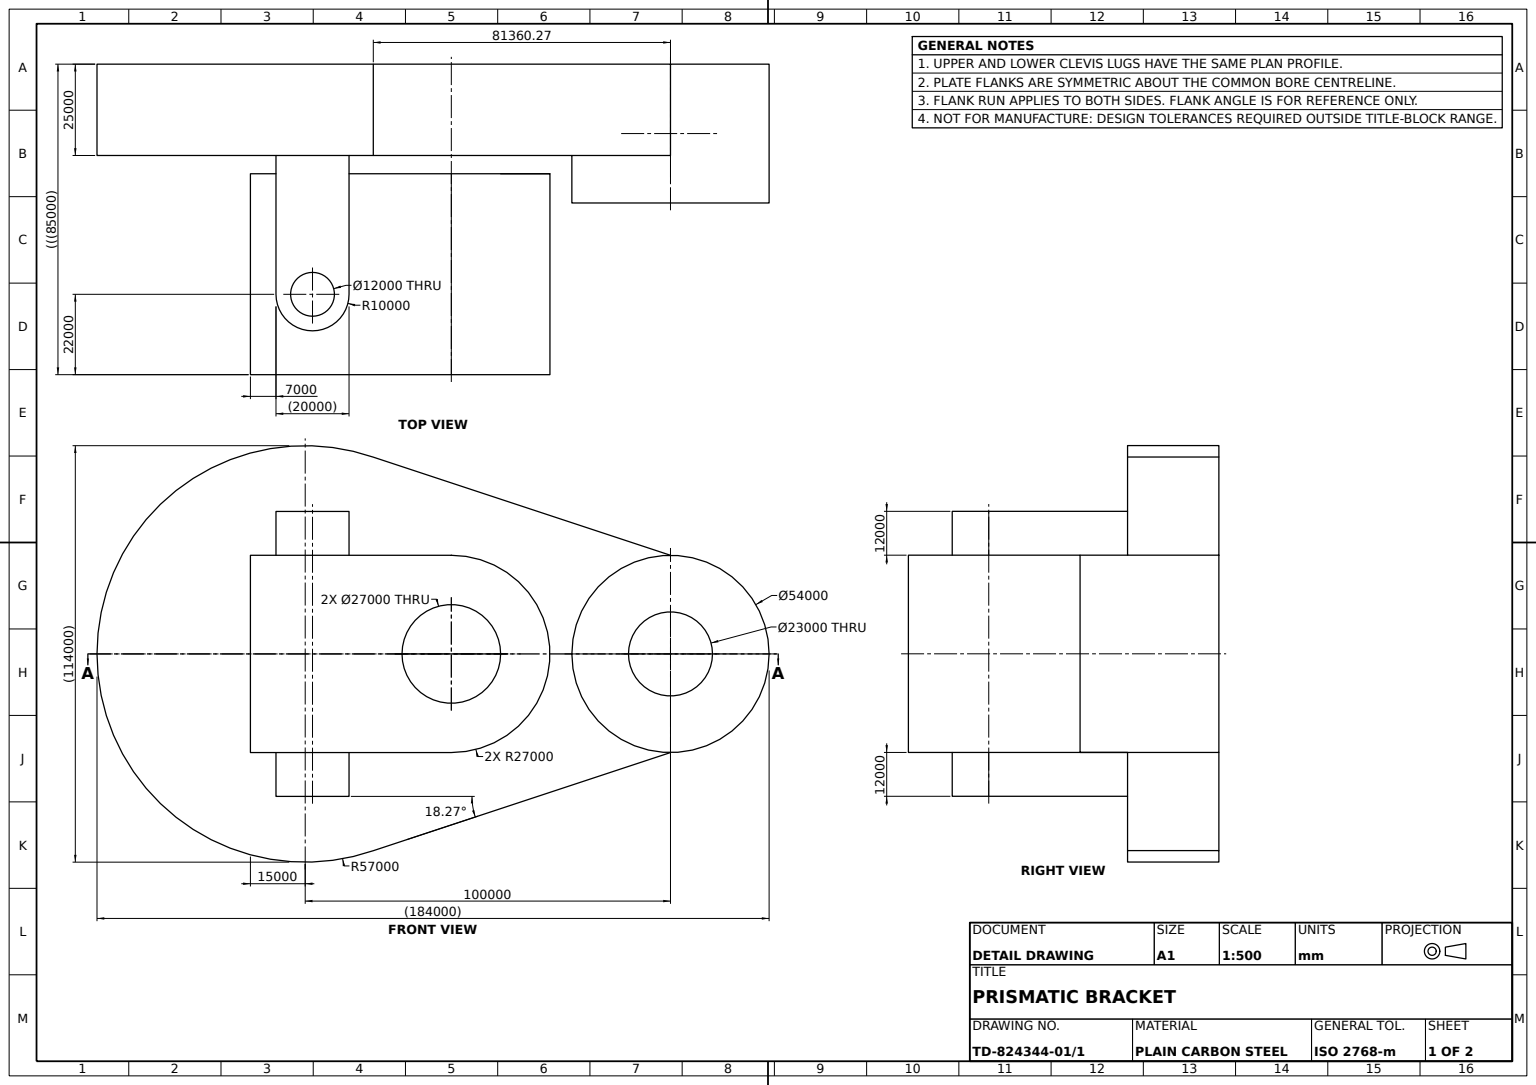
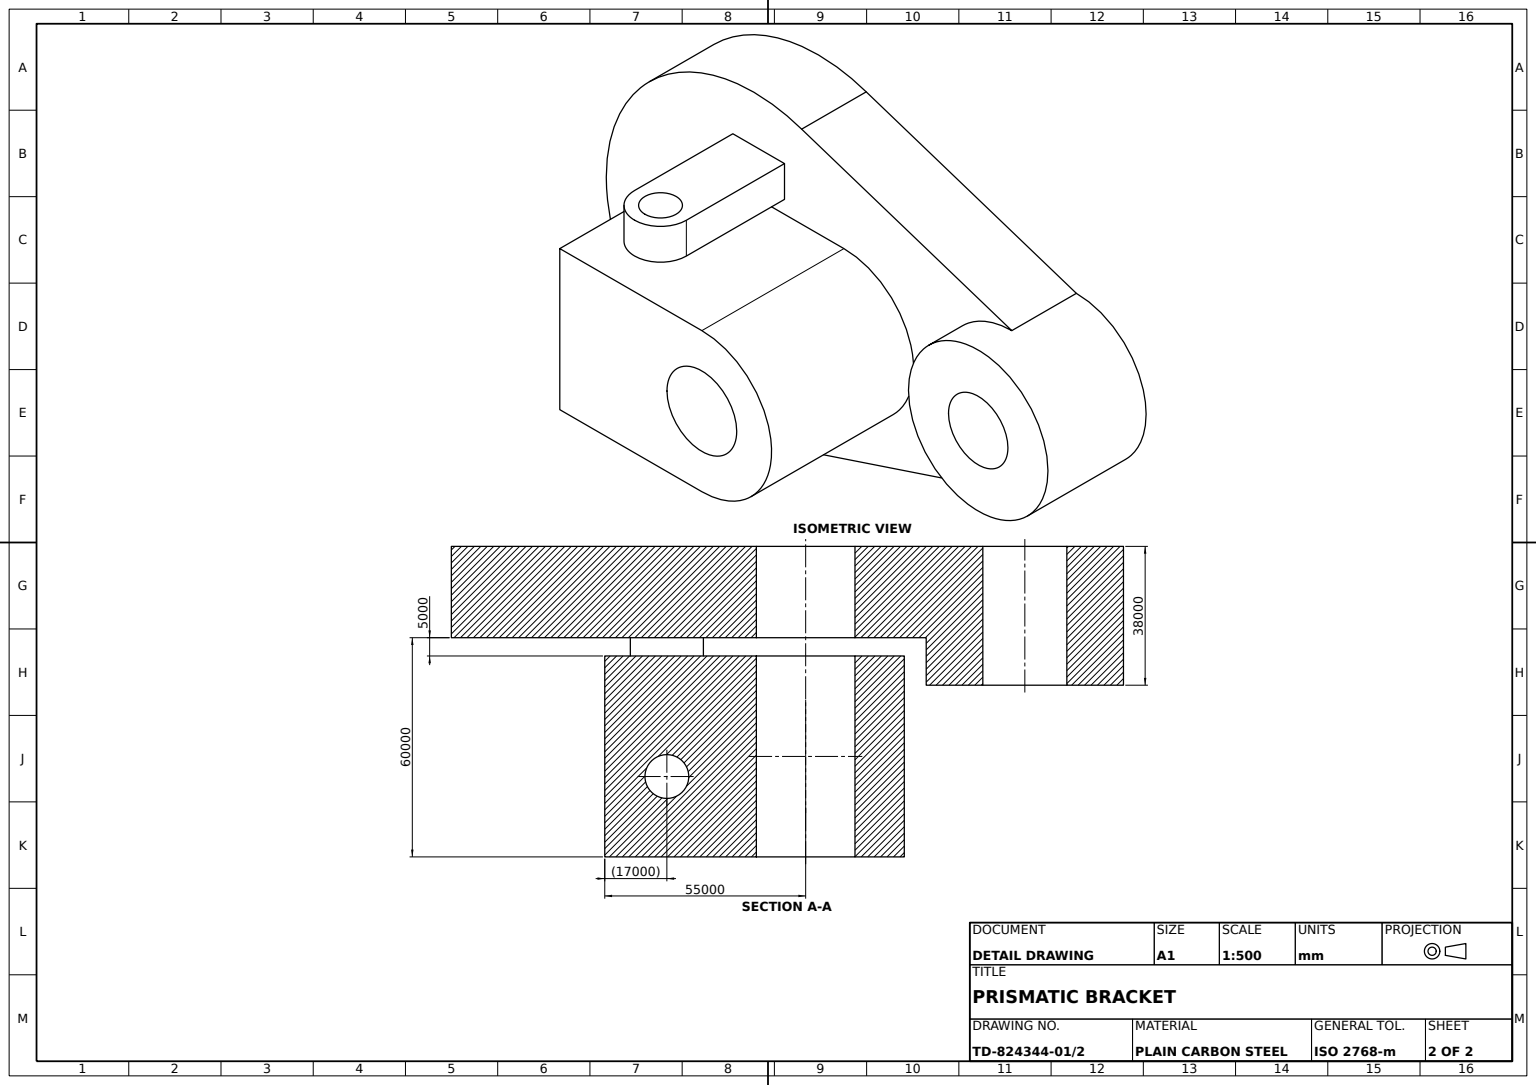
from build123d import *

# Parameters (mm, degrees)
HUB_SKETCH_54_R      = 27000
HUB_BOSS_54_DEPTH    = 19000
BASE_PLATE_DEPTH     = 25000
MOUNTING_BLOCK_DEPTH = 60000
PLATE_HOLE_SKETCH_R  = 13500
PLATE_HOLE_DEPTH     = 187412.312358673
HUB_BORE_SKETCH_23_R = 11500
HUB_BORE_23_DEPTH    = 173514.688220843
BLOCK_SLOT_REACH     = 166642.331
BLOCK_SLOT_SKETCH_W  = 5000
BLOCK_SLOT_SKETCH_H  = 54000
CLEVIS_LUG_1_DEPTH   = 12000
CLEVIS_LUG_2_DEPTH   = 12000
PIN_HOLE_SKETCH_12_R = 6000
PIN_HOLE_12_DEPTH    = 195502.918149158


with BuildPart() as part:
    # Hub Sketch Ø54 → Hub Boss Ø54 (new, symmetric)
    with BuildSketch(Plane.XY):
        Circle(HUB_SKETCH_54_R)
    extrude(amount=HUB_BOSS_54_DEPTH, both=True)

    # Base Plate Sketch → Base Plate (add)
    with BuildSketch(Plane.XY.offset(19000)):
        with BuildLine():
            Line((0, 27000), (81360.266783536, 53866.133568496))
            ThreePointArc((81360.266783536, 53866.133568496), (157000, 0), (81360.266783536, -53866.133568496))
            Line((81360.266783536, -53866.133568496), (0, -27000))
            ThreePointArc((0, -27000), (27000, 0), (0, 27000))
        make_face()
    extrude(amount=-BASE_PLATE_DEPTH)

    # Mounting Block Sketch → Mounting Block (add)
    with BuildSketch(Plane(origin=(0, 0, -6000), x_dir=(-1, 0, 0), z_dir=(0, 0, -1))):
        with BuildLine():
            Line((-115000, 27000), (-60000, 27000))
            ThreePointArc((-60000, 27000), (-33000, 0), (-60000, -27000))
            Line((-60000, -27000), (-115000, -27000))
            Line((-115000, -27000), (-115000, 27000))
        make_face()
    extrude(amount=MOUNTING_BLOCK_DEPTH)

    # Plate Hole Sketch → Plate Hole (cut, through all)
    with BuildSketch(Plane(origin=(0, 0, -66000), x_dir=(-1, 0, 0), z_dir=(0, 0, -1))):
        with Locations((-60000, 0)):
            Circle(PLATE_HOLE_SKETCH_R)
    extrude(amount=-PLATE_HOLE_DEPTH, mode=Mode.SUBTRACT)

    # Hub Bore Sketch Ø23 → Hub Bore Ø23 (cut, through all)
    with BuildSketch(Plane(origin=(0, 0, -19000), x_dir=(-1, 0, 0), z_dir=(0, 0, -1))):
        Circle(HUB_BORE_SKETCH_23_R)
    extrude(amount=-HUB_BORE_23_DEPTH, mode=Mode.SUBTRACT)

    # Block Slot Sketch → Block Slot (cut, up to next)
    with BuildSketch(Plane(origin=(115000, 0, 0), x_dir=(0, 0, -1), z_dir=(1, 0, 0)), mode=Mode.PRIVATE) as block_slot_sk1:
        with Locations((8500, 0)):
            Rectangle(BLOCK_SLOT_SKETCH_W, BLOCK_SLOT_SKETCH_H)
    block_slot_tool1 = extrude(block_slot_sk1.sketch, amount=-BLOCK_SLOT_REACH, mode=Mode.PRIVATE) & part.part
    add(block_slot_tool1.solids().sort_by_distance((115000, 0, -8500))[0], mode=Mode.SUBTRACT)


with BuildPart() as block_slot_piece_1:
    # of the separate pieces the step leaves, piece 1, a body of its own (block_slot_pieces)
    add(part.part.solids().sort_by_distance((27000, 0, -19000))[0])



with BuildPart() as block_slot_piece_2:
    # of the separate pieces the step leaves, piece 2, a body of its own (block_slot_pieces)
    add(part.part.solids().sort_by_distance((60000, 27000, -11000))[0])


with BuildPart() as block_slot_piece_1_1:
    add(block_slot_piece_1.part)

    add(block_slot_piece_2.part)  # Clevis Lug 1 merges Block Slot piece 2
    # Clevis Lug 1 Sketch → Clevis Lug 1 (add)
    with BuildSketch(Plane.XZ.offset(27000)):
        with BuildLine():
            Line((108000, -6000), (88000, -6000))
            Line((88000, -6000), (88000, -44000))
            ThreePointArc((88000, -44000), (98000, -54000), (108000, -44000))
            Line((108000, -44000), (108000, -6000))
        make_face()
    extrude(amount=CLEVIS_LUG_1_DEPTH)

    # Clevis Lug 2 Sketch → Clevis Lug 2 (add)
    with BuildSketch(Plane(origin=(0, 27000, 0), x_dir=(1, 0, 0), z_dir=(0, 1, 0))):
        with BuildLine():
            Line((108000, 6000), (88000, 6000))
            Line((88000, 6000), (88000, 44000))
            ThreePointArc((88000, 44000), (98000, 54000), (108000, 44000))
            Line((108000, 44000), (108000, 6000))
        make_face()
    extrude(amount=CLEVIS_LUG_2_DEPTH)

    # Pin Hole Sketch Ø12 → Pin Hole Ø12 (cut, through all)
    with BuildSketch(Plane(origin=(0, 39000, 0), x_dir=(1, 0, 0), z_dir=(0, 1, 0))):
        with Locations(Location((98000, 44000, 0), (0, 0, 270))):
            Circle(PIN_HOLE_SKETCH_12_R)
    extrude(amount=-PIN_HOLE_12_DEPTH, mode=Mode.SUBTRACT)


solid = block_slot_piece_1_1.part
